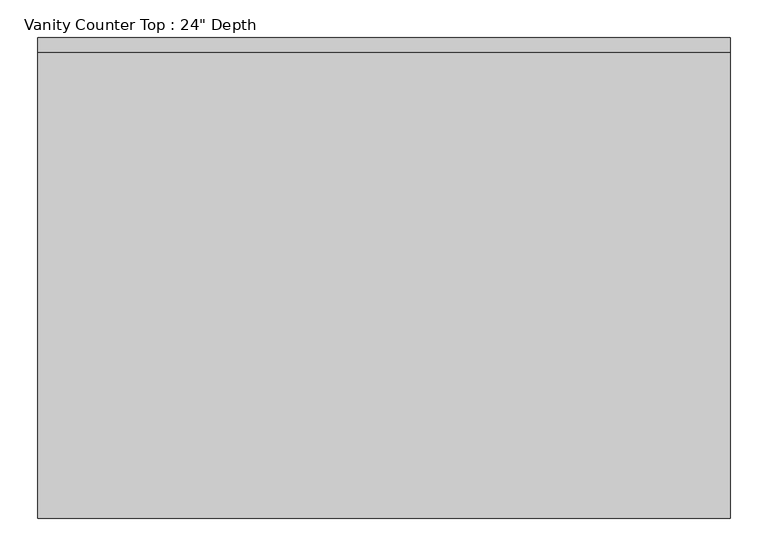
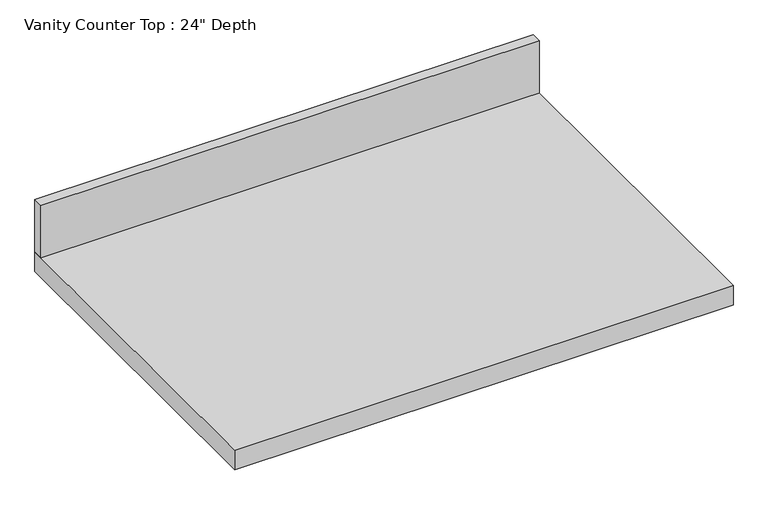
"""IFC4 building model written with IfcOpenShell, lengths in millimetres: furniture geometry."""

from ifc_helpers import new_model, si_unit, frame, origin, place, context, project, spatial, polyline, outline, extrude, source, transform, mapped, element, save


def furniture_0c89dcb9(model_context):
    return source(origin(), model_context, "Body", "SweptSolid", [
        extrude(outline(polyline([(-286.0622951, 0.0), (-286.0622951, -635.0), (-1200.4622951, -635.0), (-1200.4622951, 0.0), (-286.0622951, 0.0)])), frame((0.0, 0.0, 749.3), z_axis=(0.0, 0.0, 1.0), x_axis=(1.0, 0.0, 0.0)), (0.0, 0.0, 1.0), 38.1),
        extrude(outline(polyline([(-1200.4622951, 0.0), (-286.0622951, 0.0), (-286.0622951, -19.05), (-1200.4622951, -19.05), (-1200.4622951, 0.0)])), frame((0.0, 0.0, 787.4), z_axis=(0.0, 0.0, 1.0), x_axis=(1.0, 0.0, 0.0)), (0.0, 0.0, 1.0), 101.6),
    ])


if __name__ == "__main__":
    model = new_model("IFC4")
    model_context = context("Model", 3, world=origin())
    ifc_project = project(units=[si_unit("LENGTHUNIT", "METRE", prefix="MILLI")], contexts=[model_context])
    site = spatial("IfcSite", under=ifc_project)
    building = spatial("IfcBuilding", under=site)
    placement = place(None, origin())
    furniture_shape = furniture_0c89dcb9(model_context)
    element("IfcFurniture", 1, ObjectType="Vanity Counter Top : 24\" Depth", at=placement, inside=building, context=model_context, shape_type="MappedRepresentation", body=[
        mapped(furniture_shape, transform((0.0, 0.0, 0.0), x_axis=(1.0, 0.0, 0.0), y_axis=(0.0, 1.0, 0.0), z_axis=(0.0, 0.0, 1.0))),
    ])
    save(model, "model.ifc")

# Revit data of these elements
# Type "Vanity Counter Top : 24\" Depth"
#   Counter Thickness = 0' - 1 1/2"
#   Depth = 2' - 1"
#   Height = 2' - 7"
#   Length [instance default] = 4' - 0"
#   Counter Top Material = Counter Top
#   Default Elevation = 0
# Element 1 (IfcFurniture, "Vanity Counter Top : 24\" Depth")
#   Length = 3' - 0"
#   Materials on its faces: "Counter Top"
# Materials
#   "Counter Top": colour RGB 226 177 128, transparency 0
